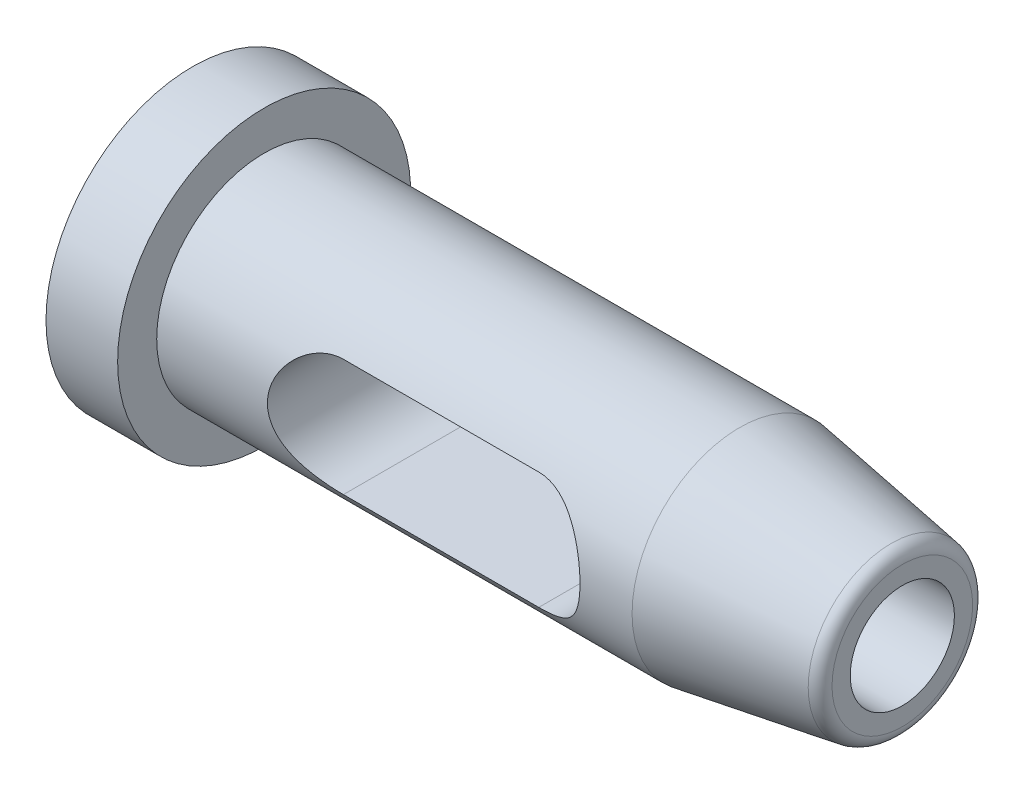
from build123d import *

# Parameters (mm, degrees)
SIDE_WINDOW_CUT_DEPTH      = 114.549548656
SIDE_WINDOW_CUT_DEPTH_BACK = 114.549548656
EDGE_FILLET_R2_R           = 2
BORE_16_REACH              = 115.55
BORE_16_END_RADIUS         = 9
BORE_SKETCH_16_R           = 8


with BuildPart() as part:
    # Holder Profile Sketch → Holder Body Revolve (revolve)
    with BuildSketch(Plane.XY, mode=Mode.PRIVATE) as holder_body_revolve_sk:
        Polygon((0, 0), (0, 22.5), (11, 22.5), (11, 16.5), (84, 16.5), (109, 12.5), (109, 0), align=None)
    revolve(holder_body_revolve_sk.sketch.rotate(Axis((-42.829787234, 0, 0), (1, 0, 0)), 90), axis=Axis((-42.829787234, 0, 0), (1, 0, 0)))

    # Side Window Sketch → Side Window Cut (cut, two sides: drawn at the far end of the back side and taken through both)
    with BuildSketch(Plane.XY.offset(-SIDE_WINDOW_CUT_DEPTH_BACK)):
        with BuildLine():
            Line((37, 9), (67, 9))
            ThreePointArc((67, 9), (76, 0), (67, -9))
            Line((67, -9), (37, -9))
            ThreePointArc((37, -9), (28, 0), (37, 9))
        make_face()
    extrude(amount=SIDE_WINDOW_CUT_DEPTH + SIDE_WINDOW_CUT_DEPTH_BACK, mode=Mode.SUBTRACT)

    # Edge Fillet R2
    edge_fillet_r2_edges = [part.edges().sort_by_distance(p)[0] for p in [
        (109, 0, -12.5),
    ]]
    fillet(edge_fillet_r2_edges, radius=EDGE_FILLET_R2_R)

    # Bore Ø16: up to this cylinder (the profile starts outside it)
    bore_16_end = Plane(origin=(67, 0, 0), z_dir=(0, 0, 1)) * Cylinder(BORE_16_END_RADIUS, 250.1, mode=Mode.PRIVATE)
    # Bore Sketch Ø16 → Bore Ø16 (cut, up to the surface)
    with BuildSketch(Plane(origin=(109, 0, 0), x_dir=(0, 0, -1), z_dir=(1, 0, 0)), mode=Mode.PRIVATE) as bore_16_sk1:
        Circle(BORE_SKETCH_16_R)
    bore_16_tool1 = extrude(bore_16_sk1.sketch, amount=-BORE_16_REACH, mode=Mode.PRIVATE) - bore_16_end
    add(bore_16_tool1.solids().sort_by_distance((109, 0, 0))[0], mode=Mode.SUBTRACT)


solid = part.part
